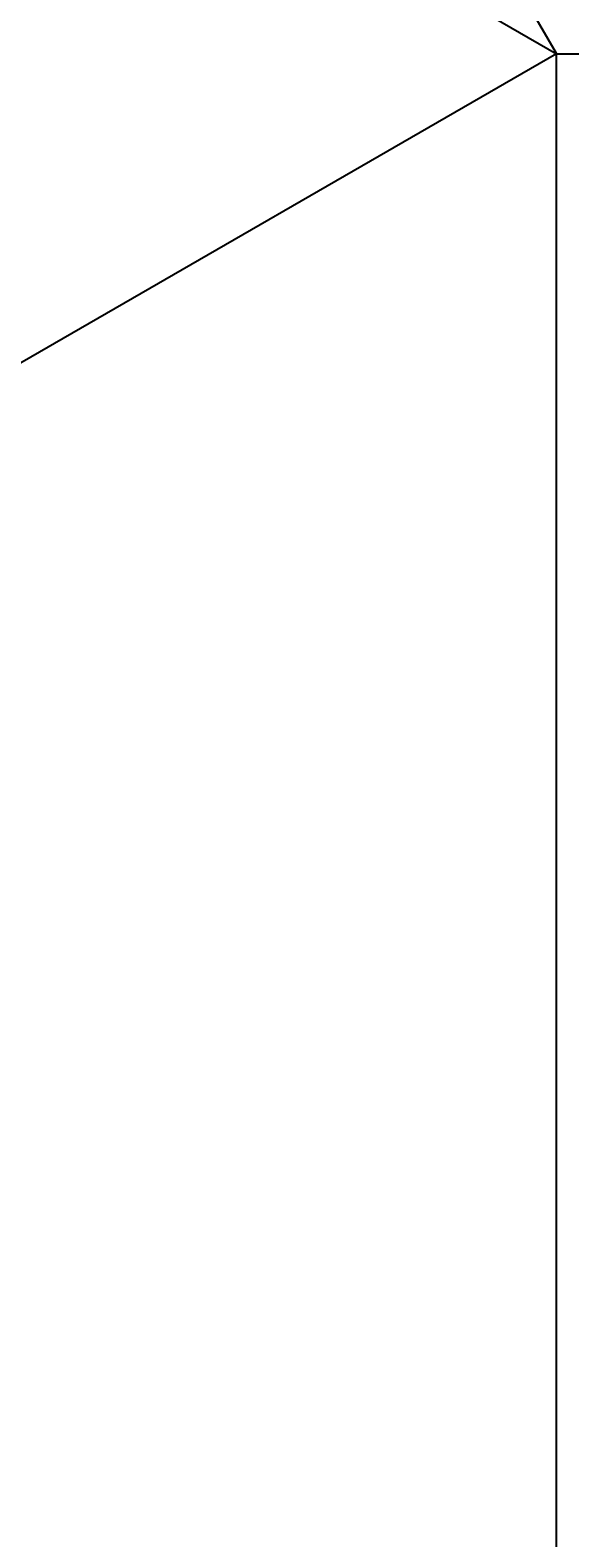
# Model space of a CAD drawing. Units: metres. Extents: x -2391 to 4922, y -635 to 4845.
# Tile 9 of 37: x -271 to 39, y 53 to 919. Entities that reach past the tile are written whole.
import ezdxf

# ---------------------------------------------------------------- set-up
doc = ezdxf.new("R2010")
doc.units = ezdxf.units.M
doc.header["$MEASUREMENT"] = 0
doc.layers.add('A-ANNO-DIMS', color=2, linetype='Continuous', lineweight=18)
doc.layers.add('A-FLOR-FIXT', color=3, linetype='Continuous', lineweight=25)
doc.styles.get("Standard").update_dxf_attribs({"font": 'arial.ttf'})
doc.dimstyles.get("Standard").update_dxf_attribs({"dimtxt": 5, "dimasz": 4, "dimexe": 0.18, "dimexo": 0.0625, "dimgap": 0.09, "dimtad": 0, "dimtih": 1, "dimtoh": 1, "dimdec": 0, "dimzin": 0, "dimdsep": 46, "dimtxsty": 'Standard', "dimcen": 0.09, "dimadec": 0, "dimazin": 0, "dimtfac": 1, "dimtdec": 0, "dimtofl": 0, "dimtmove": 0, "dimatfit": 3, "dimfxl": 1, "dimtolj": 1, "dimtzin": 0, "dimarcsym": 0})

# ---------------------------------------------------------------- blocks, each defined once
blk = doc.blocks.new('*D8')
at = {"layer": 'A-ANNO-DIMS', "color": 0, "lineweight": -2, "transparency": 16777216}
for p, q in [((-2047.33, 3005.21), (-2047.33, -631.4)), ((4577.76, 2350.21), (4577.76, -631.4)), ((-2043.33, -631.22), (1257.62, -631.22)), ((4573.76, -631.22), (1272.8, -631.22))]:
    blk.add_line(p, q, dxfattribs=at)
at = {"layer": 'A-ANNO-DIMS', "color": 0, "transparency": 16777216}
for points in [[(-2043.33, -630.56), (-2043.33, -631.89), (-2047.33, -631.22)], [(4573.76, -630.56), (4573.76, -631.89), (4577.76, -631.22)]]:
    blk.add_solid(points, dxfattribs=at)
at = {"layer": 'Defpoints', "color": 0, "transparency": 16777216}
for p in [(-2047.33, 3005.28), (4577.76, 2350.28), (4577.76, -631.22)]:
    blk.add_point(p, dxfattribs=at)
at = {"layer": 'A-ANNO-DIMS', "color": 0, "transparency": 16777216, "insert": (1265.21, -631.22), "char_height": 5, "attachment_point": 5}
blk.add_mtext('\\A1;6625', dxfattribs=at)
blk = doc.blocks.new('*D10')
at = {"layer": 'A-ANNO-DIMS', "color": 0, "lineweight": -2, "transparency": 16777216}
for p, q in [((550.68, 4505.28), (-2384.01, 4505.28)), ((-2383.83, 4501.28), (-2383.83, 2107.92)), ((-2383.83, -290.72), (-2383.83, 2102.63)), ((-488.55, -294.72), (-2384.01, -294.72))]:
    blk.add_line(p, q, dxfattribs=at)
at = {"layer": 'A-ANNO-DIMS', "color": 0, "transparency": 16777216}
for points in [[(-2384.5, 4501.28), (-2383.17, 4501.28), (-2383.83, 4505.28)], [(-2384.5, -290.72), (-2383.17, -290.72), (-2383.83, -294.72)]]:
    blk.add_solid(points, dxfattribs=at)
at = {"layer": 'Defpoints', "color": 0, "transparency": 16777216}
for p in [(-2383.83, 4505.28), (550.74, 4505.28), (-488.49, -294.72)]:
    blk.add_point(p, dxfattribs=at)
at = {"layer": 'A-ANNO-DIMS', "color": 0, "transparency": 16777216, "insert": (-2383.83, 2105.28), "char_height": 5, "attachment_point": 5}
blk.add_mtext('\\A1;4800', dxfattribs=at)
blk = doc.blocks.new('*D47')
at = {"layer": 'A-ANNO-DIMS', "color": 0, "lineweight": -2, "transparency": 16777216}
for p, q in [((31.1, 905.33), (-137.21, 1196.85)), ((-140.59, 1194.69), (-367.03, 1063.96)), ((-602.63, 927.94), (-376.18, 1058.67)), ((-437.87, 634.57), (-606.18, 926.09))]:
    blk.add_line(p, q, dxfattribs=at)
at = {"layer": 'A-ANNO-DIMS', "color": 0, "transparency": 16777216}
for points in [[(-140.92, 1195.27), (-140.25, 1194.12), (-137.12, 1196.69)], [(-602.96, 928.51), (-602.29, 927.36), (-606.09, 925.94)]]:
    blk.add_solid(points, dxfattribs=at)
at = {"layer": 'Defpoints', "color": 0, "transparency": 16777216}
for p in [(-137.12, 1196.69), (31.13, 905.28), (-437.84, 634.52)]:
    blk.add_point(p, dxfattribs=at)
at = {"layer": 'A-ANNO-DIMS', "color": 0, "transparency": 16777216, "insert": (-371.61, 1061.31), "char_height": 5, "attachment_point": 5}
blk.add_mtext('\\A1;541.5', dxfattribs=at)
blk = doc.blocks.new('*D48')
at = {"layer": 'A-ANNO-DIMS', "color": 0, "lineweight": -2, "transparency": 16777216}
for p, q in [((31.19, 905.28), (367.81, 905.28)), ((367.63, 901.28), (367.63, 457.92)), ((367.63, 9.28), (367.63, 452.63)), ((31.19, 5.28), (367.81, 5.28))]:
    blk.add_line(p, q, dxfattribs=at)
at = {"layer": 'A-ANNO-DIMS', "color": 0, "transparency": 16777216}
for points in [[(366.96, 901.28), (368.29, 901.28), (367.63, 905.28)], [(366.96, 9.28), (368.29, 9.28), (367.63, 5.28)]]:
    blk.add_solid(points, dxfattribs=at)
at = {"layer": 'Defpoints', "color": 0, "transparency": 16777216}
for p in [(31.13, 905.28), (31.13, 5.28), (367.63, 5.28)]:
    blk.add_point(p, dxfattribs=at)
at = {"layer": 'A-ANNO-DIMS', "color": 0, "transparency": 16777216, "insert": (367.63, 455.28), "char_height": 5, "attachment_point": 5}
blk.add_mtext('\\A1;900', dxfattribs=at)

msp = doc.modelspace()

# ---------------------------------------------------------------- linework, layer by layer
at = {"layer": 'A-FLOR-FIXT'}
for p, q in [((-1527.7191, 1805.2763), (31.1266, 905.2763)), ((31.1266, 905.2763), (-488.4886, 605.2763)), ((31.1266, 5.2763), (31.1266, 905.2763))]:
    msp.add_line(p, q, dxfattribs=at)

# ---------------------------------------------------------------- dimensions: what is measured, and where the dimension line sits
at = {"layer": 'A-ANNO-DIMS'}
for base, p1, p2, angle, override, picture, middle in [((-2383.8343, 4505.2763), (-488.4886, -294.7237), (550.7419, 4505.2763), 90, {"dimdec": 0, "dimlfac": 1, "dimrnd": 0, "dimzin": 0, "dimdsep": 46, "dimlunit": 2}, '*D10', (-2383.8343, 2105.2763)), ((-137.1234, 1196.6938), (-437.841, 634.5176), (31.1266, 905.2763), 30, {"dimdec": 1, "dimlfac": 1, "dimrnd": 0, "dimzin": 0, "dimdsep": 46, "dimlunit": 2}, '*D47', (-371.6072, 1061.3145)), ((367.6266, 5.2763), (31.1266, 905.2763), (31.1266, 5.2763), 270, {"dimdec": 0, "dimlfac": 1, "dimrnd": 0, "dimzin": 0, "dimdsep": 46, "dimlunit": 2}, '*D48', (367.6266, 455.2763))]:
    dim = msp.add_linear_dim(base=base, p1=p1, p2=p2, angle=angle, dimstyle='Standard', override=override, dxfattribs=at)
    dim.commit()
    dim.dimension.update_dxf_attribs({"geometry": picture, "text_midpoint": middle})
dim = msp.add_linear_dim(base=(4577.76, -631.2237), p1=(-2047.3343, 3005.2763), p2=(4577.76, 2350.2763), dimstyle='Standard', override={"dimdec": 0, "dimlfac": 1, "dimrnd": 0, "dimzin": 0, "dimdsep": 46, "dimlunit": 2}, dxfattribs=at)
dim.commit()
dim.dimension.update_dxf_attribs({"geometry": '*D8', "text_midpoint": (1265.2128, -631.2237)})

doc.saveas('drawing.dxf')
